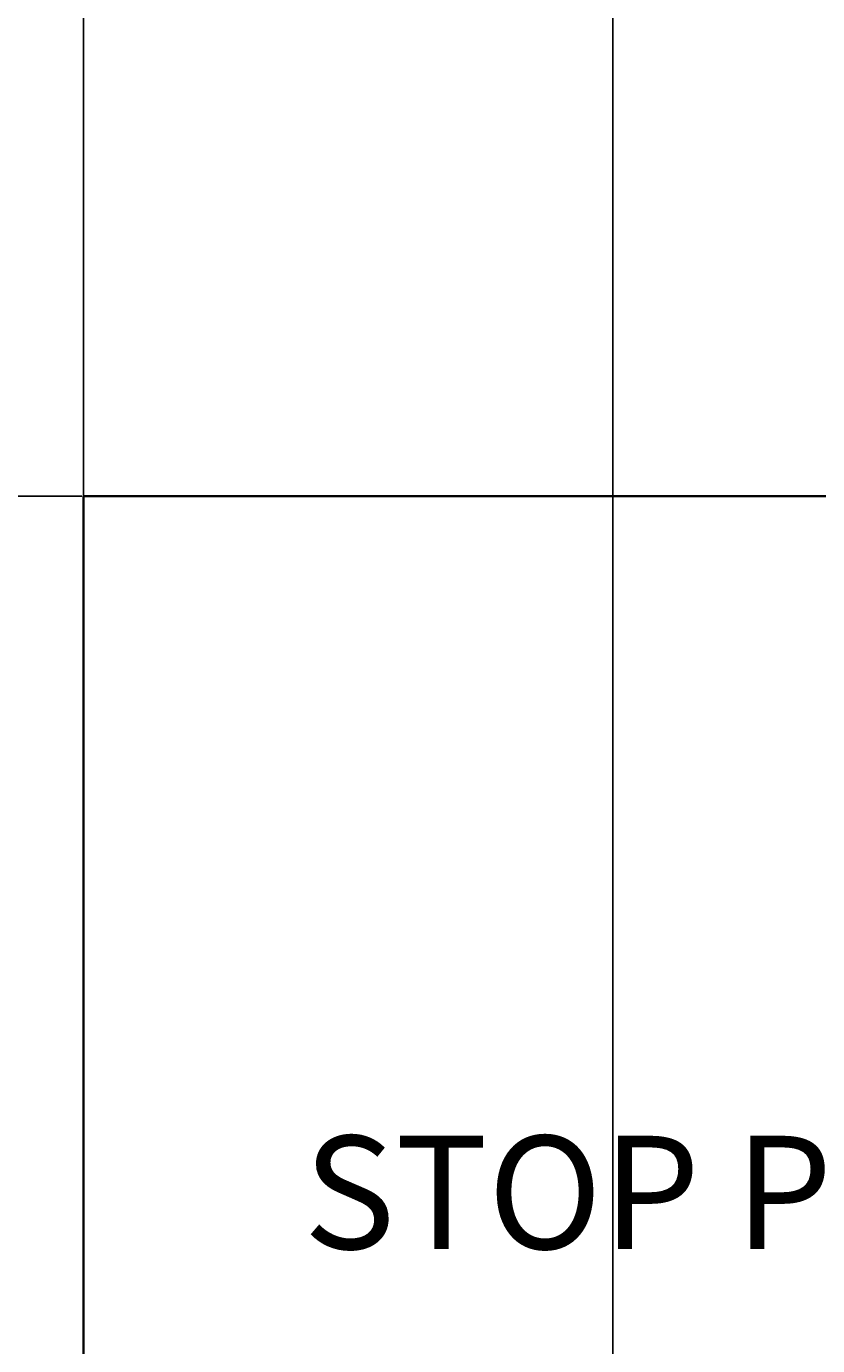
# Model space of a CAD drawing. Units: inches. Extents: x 738 to 1068, y 378 to 757.
# Tile 36 of 41: x 779 to 809, y 655 to 704. Entities that reach past the tile are written whole.
import ezdxf

# ---------------------------------------------------------------- set-up
doc = ezdxf.new("R2010")
doc.units = ezdxf.units.IN
doc.header["$MEASUREMENT"] = 0
for name, color, linetype, lineweight in [('A-ANNO-DIMS', 2, 'Continuous', 18), ('E-ANNO-TEXT', 7, 'Continuous', 18), ('E-POWR-FEED', 7, 'Continuous', 35)]:
    doc.layers.add(name, color=color, linetype=linetype, lineweight=lineweight)
doc.styles.get("Standard").update_dxf_attribs({"font": 'arial.ttf'})
doc.dimstyles.get("Standard").update_dxf_attribs({"dimtxt": 0.18, "dimasz": 0.18, "dimexe": 0.18, "dimexo": 0.0625, "dimgap": 0.09, "dimtad": 0, "dimtih": 1, "dimtoh": 1, "dimdec": 4, "dimzin": 0, "dimdsep": 46, "dimtxsty": 'Standard', "dimcen": 0.09, "dimadec": 0, "dimazin": 0, "dimtfac": 1, "dimtdec": 4, "dimtofl": 0, "dimtmove": 0, "dimatfit": 3, "dimfxl": 1, "dimtolj": 1, "dimtzin": 0, "dimarcsym": 0})

# ---------------------------------------------------------------- blocks, each defined once
blk = doc.blocks.new('*D24')
at = {"layer": 'A-ANNO-DIMS', "color": 0, "lineweight": -2, "transparency": 16777216}
for p, q in [((781.427, 686.329), (738.194, 686.329)), ((738.374, 686.149), (738.374, 666.839)), ((738.374, 647.165), (738.374, 666.475)), ((781.427, 646.985), (738.194, 646.985))]:
    blk.add_line(p, q, dxfattribs=at)
at = {"layer": 'A-ANNO-DIMS', "color": 0, "transparency": 16777216}
for points in [[(738.344, 686.149), (738.404, 686.149), (738.374, 686.329)], [(738.344, 647.165), (738.404, 647.165), (738.374, 646.985)]]:
    blk.add_solid(points, dxfattribs=at)
at = {"layer": 'Defpoints', "color": 0, "transparency": 16777216}
for p in [(738.374, 686.329), (781.49, 686.329), (781.49, 646.985)]:
    blk.add_point(p, dxfattribs=at)
at = {"layer": 'A-ANNO-DIMS', "color": 0, "transparency": 16777216, "insert": (738.374, 666.657), "char_height": 0.18, "attachment_point": 5}
blk.add_mtext('\\A1;39.34', dxfattribs=at)
blk = doc.blocks.new('*D31')
at = {"layer": 'A-ANNO-DIMS', "color": 0, "lineweight": -2, "transparency": 16777216}
for p, q in [((781.49, 531.463), (781.49, 756.505)), ((781.67, 756.325), (790.802, 756.325)), ((800.842, 756.325), (791.71, 756.325)), ((801.022, 531.463), (801.022, 756.505))]:
    blk.add_line(p, q, dxfattribs=at)
at = {"layer": 'A-ANNO-DIMS', "color": 0, "transparency": 16777216}
for points in [[(781.67, 756.355), (781.67, 756.295), (781.49, 756.325)], [(800.842, 756.355), (800.842, 756.295), (801.022, 756.325)]]:
    blk.add_solid(points, dxfattribs=at)
at = {"layer": 'Defpoints', "color": 0, "transparency": 16777216}
for p in [(801.022, 756.325), (781.49, 531.401), (801.022, 531.401)]:
    blk.add_point(p, dxfattribs=at)
at = {"layer": 'A-ANNO-DIMS', "color": 0, "transparency": 16777216, "insert": (791.256, 756.325), "char_height": 0.18, "attachment_point": 5}
blk.add_mtext('\\A1;19.532', dxfattribs=at)
blk = doc.blocks.new('*D34')
at = {"layer": 'A-ANNO-DIMS', "color": 0, "lineweight": -2, "transparency": 16777216}
for p, q in [((781.49, 686.266), (781.49, 378.239)), ((830.489, 686.266), (830.489, 378.239)), ((781.67, 378.419), (805.767, 378.419)), ((830.309, 378.419), (806.212, 378.419))]:
    blk.add_line(p, q, dxfattribs=at)
at = {"layer": 'A-ANNO-DIMS', "color": 0, "transparency": 16777216}
for points in [[(781.67, 378.449), (781.67, 378.389), (781.49, 378.419)], [(830.309, 378.449), (830.309, 378.389), (830.489, 378.419)]]:
    blk.add_solid(points, dxfattribs=at)
at = {"layer": 'Defpoints', "color": 0, "transparency": 16777216}
for p in [(781.49, 686.329), (830.489, 686.329), (830.489, 378.419)]:
    blk.add_point(p, dxfattribs=at)
at = {"layer": 'A-ANNO-DIMS', "color": 0, "transparency": 16777216, "insert": (805.99, 378.419), "char_height": 0.18, "attachment_point": 5}
blk.add_mtext('\\A1;49', dxfattribs=at)

msp = doc.modelspace()

# ---------------------------------------------------------------- linework, layer by layer
at = {"layer": 'E-POWR-FEED'}
for p, q in [((826.2488, 686.329), (781.4897, 686.329)), ((781.4897, 686.329), (781.4897, 437.7164))]:
    msp.add_line(p, q, dxfattribs=at)

# ---------------------------------------------------------------- texts
at = {"layer": 'E-ANNO-TEXT'}
msp.add_text('STOP PLC SYSTEM', height=4.175074, dxfattribs=at).set_placement((789.5941, 658.5662))

# ---------------------------------------------------------------- dimensions: what is measured, and where the dimension line sits
at = {"layer": 'A-ANNO-DIMS'}
for base, p1, p2, override, picture, middle in [((801.0218, 756.3251), (781.4897, 531.4009), (801.0218, 531.4009), {"dimdec": 3, "dimlfac": 1, "dimrnd": 0, "dimzin": 0, "dimdsep": 46, "dimlunit": 2}, '*D31', (791.2557, 756.3251)), ((830.4893, 378.4191), (781.4897, 686.329), (830.4893, 686.329), {"dimdec": 0, "dimlfac": 1, "dimrnd": 0, "dimzin": 0, "dimdsep": 46, "dimlunit": 2}, '*D34', (805.9895, 378.4191))]:
    dim = msp.add_linear_dim(base=base, p1=p1, p2=p2, dimstyle='Standard', override=override, dxfattribs=at)
    dim.commit()
    dim.dimension.update_dxf_attribs({"geometry": picture, "text_midpoint": middle})
dim = msp.add_linear_dim(base=(738.3736, 686.329), p1=(781.4897, 646.9853), p2=(781.4897, 686.329), angle=90, dimstyle='Standard', override={"dimdec": 2, "dimlfac": 1, "dimrnd": 0, "dimzin": 0, "dimdsep": 46, "dimlunit": 2}, dxfattribs=at)
dim.commit()
dim.dimension.update_dxf_attribs({"geometry": '*D24', "text_midpoint": (738.3736, 666.6571)})

doc.saveas('drawing.dxf')
